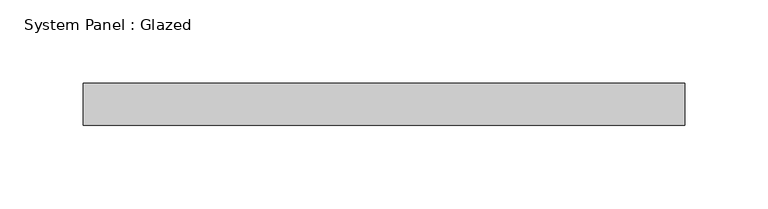
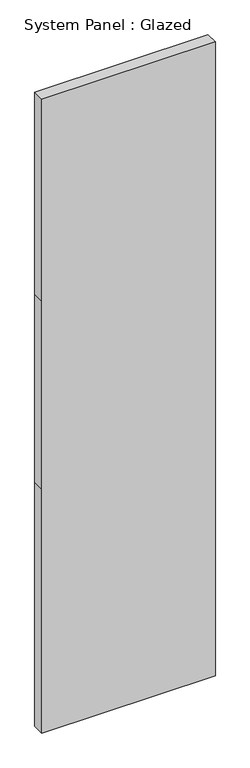
"""IFC4 building model written with IfcOpenShell, lengths in millimetres: plate geometry, System Panel : Glazed."""

from ifc_helpers import new_model, si_unit, frame, origin, place, context, project, spatial, polyline, outline, extrude, source, transform, mapped, element, save


def system_panel_glazed_22d47ebb(model_context):
    return source(origin(), model_context, "Body", "SweptSolid", [
        extrude(outline(polyline([(0.0, -180.975), (0.0, 180.975), (537.6333333, 180.975), (952.5, 180.975), (1397.0, 180.975), (1397.0, -180.975), (952.5, -180.975), (537.6333333, -180.975), (0.0, -180.975)])), frame((0.0, 19.05, 0.0), z_axis=(0.0, 1.0, 0.0), x_axis=(0.0, 0.0, 1.0)), (0.0, 0.0, 1.0), 25.4),
    ])


if __name__ == "__main__":
    model = new_model("IFC4")
    model_context = context("Model", 3, world=origin())
    ifc_project = project(units=[si_unit("LENGTHUNIT", "METRE", prefix="MILLI")], contexts=[model_context])
    site = spatial("IfcSite", under=ifc_project)
    building = spatial("IfcBuilding", under=site)
    placement = place(None, origin())
    system_panel_glazed_shape = system_panel_glazed_22d47ebb(model_context)
    element("IfcPlate", 1, ObjectType="System Panel : Glazed", at=placement, inside=building, context=model_context, shape_type="MappedRepresentation", body=[
        mapped(system_panel_glazed_shape, transform((0.0, 0.0, 0.0), x_axis=(1.0, 0.0, 0.0), y_axis=(0.0, 1.0, 0.0), z_axis=(0.0, 0.0, 1.0))),
    ])
    save(model, "model.ifc")

# Revit data of these elements
# Type "System Panel : Glazed"
#   Construction Type Id = "GSP4R"
#   Analytic Construction = "1/8 in Pilkington single glazing"
#   Visual Light Transmittance = 0.9
#   Solar Heat Gain Coefficient = 0.86
#   Heat Transfer Coefficient (U) = 1.18115 BTU/(h·ft²·°F)
#   Define Thermal Properties by = 1
# Element 1 (IfcPlate, "System Panel : Glazed")
#   Materials on its faces: "Glass"
# Materials
#   "Glass": class "Glass", colour RGB 0 128 192, transparency 0.75, Description = "Soda Lime Glass", Cost = 0
